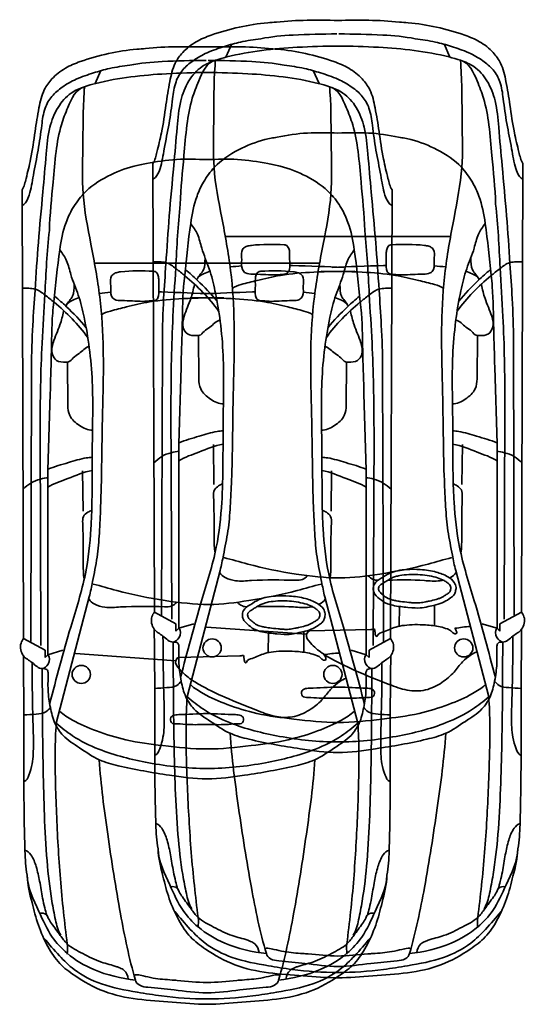
# Model space of a CAD drawing. Units: inches. Extents: x -24887 to 3061, y 1794 to 4919553.
# Tile 14 of 14: x -24887 to -22520, y 4914938 to 4919553. Entities that reach past the tile are written whole.
import ezdxf

# ---------------------------------------------------------------- set-up
doc = ezdxf.new("R2010")
doc.units = ezdxf.units.IN
doc.layers.add('door', color=4, linetype='Continuous', lineweight=25)
doc.layers.add('wall', color=7, linetype='Continuous', lineweight=35)

# ---------------------------------------------------------------- blocks, each defined once
blk = doc.blocks.new('A$C242571DA')
for p, q in [((1659.9, 1632), (1714.3, 1732.5)), ((1714.3, 1732.5), (3817.1, 1739.9)), ((1699.9, 1699.4), (2984.7, 1695.8)), ((1638.3, 1618.5), (1625.1, 1632)), ((1625.1, 1632), (1659.9, 1632)), ((1638.3, 1618.5), (2503.3, 1618.5)), ((1659.9, 1548.1), (1638.3, 1618.5)), ((1681.8, 1651.6), (2695.2, 1655.3)), ((2503.3, 1618.5), (2861.6, 1607.5)), ((1317.4, 1579.7), (1909.8, 1424.9)), ((3007.2, 1526.5), (2808.1, 1525.2)), ((1644, 1489.1), (1610.4, 1020.2)), ((2311.9, 1454.3), (2500.6, 1456.9)), ((3474.6, 1401.1), (3474.6, 843)), ((4315.2, 1398), (4377.3, 1370.5)), ((1626.1, 1006.5), (1632.8, 719.7)), ((3474.6, 345.6), (3474.6, 903.8)), ((1740.2, 584.9), (1649.3, 586.9)), ((1746.1, 420.6), (1649.3, 420.6)), ((4315.2, 348.7), (4377.3, 376.3)), ((1317.4, 167), (1909.8, 321.9)), ((2311.9, 292.5), (2500.6, 289.8)), ((1659.9, 198.7), (1638.3, 128.2)), ((3007.2, 220.3), (2808.1, 221.6)), ((2503.3, 128.2), (2861.6, 139.2)), ((1638.3, 128.2), (1625.1, 114.7)), ((1625.1, 114.7), (1659.9, 114.7)), ((1638.3, 128.2), (2503.3, 128.2)), ((1659.9, 114.7), (1714.3, 14.2)), ((1681.8, 95.1), (2695.2, 91.4)), ((1699.9, 47.3), (2984.7, 51)), ((1714.3, 14.2), (3817.1, 6.9))]:
    blk.add_line(p, q)
for centre in [(1546.4, 1462.5), (1546.4, 284.2)]:
    blk.add_ellipse(centre, major_axis=(0, 42.9), ratio=0.983266, start_param=4.712389, end_param=10.995574)
for points, knots in [([(0, 873.4), (0, 927.8), (15.6, 1088.6), (25.5, 1309.8), (120.7, 1476.4), (189.2, 1569), (273.5, 1623.1), (369.9, 1666.3), (483, 1694.7), (561.3, 1714.9), (604.6, 1715.7)], [0, 0, 0, 0, 0.16039, 0.479033, 0.632967, 0.722015, 0.817474, 0.927562, 1.03733, 1.167094, 1.167094, 1.167094, 1.167094]), ([(604.6, 1715.7), (545.5, 1714.5), (448.5, 1664.6), (320.8, 1610.6), (225.4, 1521.2), (147.3, 1390.5), (121.7, 1275.2), (113.6, 1208.7)], [0, 0, 0, 0, 0.1772572, 0.3124951, 0.4151678, 0.5597243, 0.7575412, 0.7575412, 0.7575412, 0.7575412]), ([(722.7, 1726.6), (720.8, 1714.9), (694.5, 1689.9), (643, 1671.8), (573.6, 1655.4), (508.5, 1647), (455.2, 1634.7), (428.7, 1627.3), (416.9, 1624.1)], [0, 0, 0, 0, 0.034703, 0.0959761, 0.1659336, 0.2471559, 0.2929944, 0.3295918, 0.3295918, 0.3295918, 0.3295918]), ([(604.6, 1715.7), (642.1, 1723.4), (788.5, 1729.2), (1039.3, 1732.2), (1344.5, 1729.9), (1542, 1733.1), (1633.8, 1733.7)], [0, 0, 0, 0, 0.114897, 0.437061, 0.754269, 1.029686, 1.029686, 1.029686, 1.029686]), ([(1043.6, 1729.2), (1048.6, 1717.9), (1080.9, 1704.2), (1138.6, 1687.6), (1237.7, 1685.6), (1394.7, 1691.3), (1521.7, 1692.4), (1601.5, 1692.7)], [0, 0, 0, 0, 0.0364992, 0.0923739, 0.1867837, 0.3273982, 0.5667068, 0.5667068, 0.5667068, 0.5667068]), ([(1356.8, 1732.2), (1357.1, 1712.8), (1360, 1678.8), (1363.9, 1630.5), (1383.3, 1613.5), (1391, 1607.2)], [0, 0, 0, 0, 1.462159, 2.651105, 3.386321, 3.386321, 3.386321, 3.386321]), ([(1714.3, 1732.5), (1707.7, 1737.6), (1683.3, 1753), (1628.7, 1741.2), (1605.6, 1691.5), (1561.7, 1652.4), (1594.1, 1610.3), (1627.9, 1608.3), (1638.3, 1618.5)], [0, 0, 0, 0, 0.024864, 0.0846267, 0.1362471, 0.1900683, 0.2245199, 0.2681841, 0.2681841, 0.2681841, 0.2681841]), ([(2414.7, 1735), (2424.9, 1723.3), (2447.2, 1698.8), (2461.2, 1657.6), (2468.1, 1629), (2468, 1616.1)], [1.808086, 1.808086, 1.808086, 1.808086, 2.918874, 4.131288, 5.10151, 5.10151, 5.10151, 5.10151]), ([(3356.5, 1739.4), (3354.9, 1719.2), (3360.8, 1678.2), (3324, 1631.5), (3255.4, 1544.3), (3187.1, 1476.2), (3125.2, 1432.2)], [0, 0, 0, 0, 0.0597371, 0.1139981, 0.1672498, 0.3938869, 0.3938869, 0.3938869, 0.3938869]), ([(3745.3, 1736.8), (3748.5, 1730.1), (3764.2, 1717.1), (3811.5, 1698.6), (3894.7, 1686.7), (4002.9, 1663.2), (4107.9, 1648.7), (4195.8, 1638.3), (4258.6, 1603.2), (4302.1, 1549.7), (4339.9, 1483.8), (4365.2, 1407.6), (4389.6, 1324.4), (4397.9, 1266.9), (4401.8, 1235.2)], [0, 0, 0, 0, 0.0219205, 0.0572122, 0.1522539, 0.2718866, 0.3894011, 0.4710097, 0.5346344, 0.5986698, 0.6733118, 0.758696, 0.8351341, 0.9293726, 0.9293726, 0.9293726, 0.9293726]), ([(3817.1, 1739.9), (3833.2, 1729.7), (3882.9, 1718.2), (3973.3, 1695.2), (4085.1, 1680.5), (4193.8, 1662.8), (4280.6, 1644.3), (4343.9, 1598.1), (4390, 1540.3), (4427.4, 1448.7), (4457.8, 1336.6), (4475.7, 1233.4), (4478.4, 1175.1), (4479.3, 1161.6)], [0, 0, 0, 0, 0.056668, 0.14946, 0.28161, 0.392935, 0.481686, 0.542967, 0.622845, 0.69797, 0.833643, 0.965665, 1.00577, 1.00577, 1.00577, 1.00577]), ([(2984.7, 1695.8), (3051, 1695.6), (3172.1, 1691.3), (3367.4, 1677.6), (3575.2, 1664.3), (3788.2, 1643.6), (3968, 1628.1), (4103.8, 1616.8), (4203.6, 1578.1), (4271.8, 1519.5), (4300.6, 1452.1), (4341.7, 1305.3), (4361.8, 1111.2), (4367.5, 936.8), (4367.5, 873.4)], [0, 0, 0, 0, 0.198873, 0.363323, 0.587433, 0.823543, 1.004622, 1.129816, 1.230113, 1.320655, 1.388577, 1.443334, 1.771447, 1.958652, 1.958652, 1.958652, 1.958652]), ([(310.7, 1637.3), (282.5, 1613.7), (230.1, 1569.9), (148.7, 1486.2), (84.8, 1361.3), (60, 1219), (32.6, 1054.3), (25.1, 944.9), (25.1, 873.4)], [0, 0, 0, 0, 0.1095129, 0.2035347, 0.3452507, 0.5161382, 0.6275464, 0.8383798, 0.8383798, 0.8383798, 0.8383798]), ([(426.8, 1656.7), (428.5, 1646.6), (426.9, 1625), (399.8, 1616.6), (368.1, 1593.9), (328, 1564.6), (271.6, 1523.9), (237, 1451.9), (196.2, 1376.7), (183.8, 1314.9), (170, 1279.6), (157.2, 1254.2), (133.3, 1244.4), (118.6, 1242.9)], [0, 0, 0, 0, 0.0304541, 0.0502818, 0.0786089, 0.1479133, 0.1986294, 0.2831705, 0.3780326, 0.4523267, 0.4667809, 0.4902599, 0.5347198, 0.5347198, 0.5347198, 0.5347198]), ([(323.7, 1557.5), (344.8, 1571.9), (400.4, 1585.1), (516, 1606.8), (680.3, 1625.8), (885.4, 1635.7), (1116.8, 1642.2), (1346.1, 1644.2), (1504.7, 1644.7), (1574, 1645.7)], [0, 0, 0, 0, 0.076148, 0.165903, 0.355672, 0.569871, 0.782325, 1.050047, 1.257936, 1.257936, 1.257936, 1.257936]), ([(1555.2, 1617.8), (1527.7, 1617.8), (1472.5, 1620.4), (1392.7, 1608.8), (1318.5, 1591), (1249.4, 1545.5), (1201.4, 1466.7), (1142.8, 1385.7), (1104.8, 1240.4), (1076, 1072.3), (1056.4, 932.4), (1056.4, 873.4)], [0, 0, 0, 0, 0.082256, 0.165174, 0.241383, 0.30939, 0.405348, 0.511507, 0.603349, 0.843635, 1.017671, 1.017671, 1.017671, 1.017671]), ([(1574, 1645.7), (1572.9, 1638), (1574.1, 1622), (1559.9, 1618.7), (1555.2, 1617.8)], [0, 0, 0, 0, 0.02274132, 0.03717479, 0.03717479, 0.03717479, 0.03717479]), ([(2424, 1618.7), (2441.5, 1589.9), (2464.2, 1518.9), (2495.4, 1450.9), (2501.6, 1411.3)], [0, 0, 0, 0, 0.1000351, 0.2184418, 0.2184418, 0.2184418, 0.2184418]), ([(2507.7, 1618.4), (2521, 1587.7), (2536.6, 1527.1), (2559.6, 1458.5), (2563.3, 1420.6), (2563.8, 1411.4)], [0, 0, 0, 0, 2.528586, 4.711885, 5.408215, 5.408215, 5.408215, 5.408215]), ([(2695.2, 1655.3), (2829.9, 1655.3), (3041.2, 1651.4), (3351.3, 1630.7), (3527.5, 1623.2), (3626.6, 1612)], [0, 0, 0, 0, 0.4042759, 0.6333827, 0.9326252, 0.9326252, 0.9326252, 0.9326252]), ([(1317.4, 1579.7), (1227.8, 1586.1), (1036, 1584.8), (741.2, 1572.5), (486.1, 1553.3), (333.3, 1534.3), (283.3, 1528.5)], [0, 0, 0, 0, 0.269375, 0.574535, 0.885339, 1.036319, 1.036319, 1.036319, 1.036319]), ([(1317.4, 1579.7), (1296.6, 1555.5), (1247.9, 1494.4), (1177.6, 1350.5), (1124.2, 1137.4), (1105.5, 964.9), (1105.5, 873.4)], [0, 0, 0, 0, 0.0947759, 0.2311242, 0.4700259, 0.7400315, 0.7400315, 0.7400315, 0.7400315]), ([(3535.9, 1563.1), (3520.1, 1550.9), (3484.4, 1526.1), (3408.2, 1510.9), (3323.4, 1473.1), (3207.9, 1445), (3072.6, 1422.2), (2866.9, 1404.6), (2626.4, 1412.9), (2396.7, 1410.8), (2200.9, 1416.9), (2001.3, 1438.2), (1732.1, 1525.9), (1527.9, 1578.9), (1407.5, 1610.7)], [0, 0, 0, 0, 0.05975, 0.126928, 0.230034, 0.336675, 0.482225, 0.641324, 0.954906, 1.203173, 1.330375, 1.542773, 1.802261, 2.175545, 2.175545, 2.175545, 2.175545]), ([(2861.6, 1607.5), (2921.1, 1607.3), (3047.2, 1600.8), (3191.4, 1602), (3356.6, 1584.1), (3498.3, 1570.6), (3623.2, 1549.4), (3664.1, 1533.3)], [0, 0, 0, 0, 0.1783018, 0.3787173, 0.431954, 0.6762374, 0.8077184, 0.8077184, 0.8077184, 0.8077184]), ([(3248.1, 1545.2), (3226.9, 1550.4), (3176.1, 1562.1), (3113.7, 1592.9), (3052.6, 1605.3), (3010.4, 1578.8), (3010.3, 1545.3), (3010.3, 1515.9), (3033.7, 1500.1), (3052.6, 1465.2), (3078.9, 1443.5), (3084, 1424.4)], [0, 0, 0, 0, 0.0655106, 0.1550445, 0.2094604, 0.2438604, 0.287164, 0.3001388, 0.3275984, 0.3616951, 0.4200969, 0.4200969, 0.4200969, 0.4200969]), ([(3319, 1587.1), (3303.3, 1568.1), (3256.9, 1516.7), (3206.7, 1467.3), (3171.4, 1439.5)], [0, 0, 0, 0, 1.868162, 5.271297, 5.271297, 5.271297, 5.271297]), ([(3626.6, 1612), (3702.5, 1609.1), (3826.2, 1596.8), (3991.4, 1583.2), (4111.7, 1562.4), (4212.2, 1522.7), (4290.4, 1488), (4300.7, 1447.5)], [0, 0, 0, 0, 0.2277977, 0.3719478, 0.4996814, 0.5863441, 0.709615, 0.709615, 0.709615, 0.709615]), ([(1372.8, 1563.1), (1357.2, 1545), (1321.6, 1490.1), (1277, 1385.7), (1232.8, 1244.2), (1211.1, 1069.4), (1196.8, 942.4), (1196.8, 873.4)], [0, 0, 0, 0, 0.0708922, 0.1925846, 0.3348457, 0.5072814, 0.7109928, 0.7109928, 0.7109928, 0.7109928]), ([(2808.1, 1525.2), (2791.9, 1525.1), (2751.9, 1519.7), (2710.6, 1472.6), (2690, 1431.1), (2690.5, 1409.6)], [0, 0, 0, 0, 0.0486628, 0.1144515, 0.1777721, 0.1777721, 0.1777721, 0.1777721]), ([(3275.5, 1532.8), (3287.5, 1528.3), (3299.8, 1504.9), (3308.4, 1482.5), (3311.7, 1472.6)], [0, 0, 0, 0, 0.983949, 1.771691, 1.771691, 1.771691, 1.771691]), ([(3372.2, 1495.3), (3354.4, 1496.8), (3316, 1494.7), (3291.6, 1525.8), (3275.5, 1532.8)], [0, 0, 0, 0, 0.0535488, 0.1060573, 0.1060573, 0.1060573, 0.1060573]), ([(3664.1, 1533.3), (3687, 1526), (3734.8, 1502.3), (3816.7, 1444.8), (3884.1, 1342.9), (3925.1, 1239.9), (3937.3, 1177), (3940.4, 1157.6)], [0, 0, 0, 0, 0.0720749, 0.1581284, 0.2958089, 0.4262456, 0.4842292, 0.4842292, 0.4842292, 0.4842292]), ([(1909.8, 1424.9), (1933.5, 1418.7), (1995.6, 1407.6), (2094.4, 1385.8), (2211.8, 1377.1), (2419, 1366.9), (2704.7, 1366.5), (3032.7, 1354.2), (3316.2, 1371), (3558.7, 1415.9), (3789.1, 1461.7), (4028.9, 1452.9), (4196.2, 1455.2), (4292.7, 1447.9), (4300.7, 1447.5)], [0, 0, 0, 0, 0.073325, 0.188896, 0.303039, 0.425821, 0.811242, 1.159737, 1.41058, 1.660623, 1.899627, 2.11145, 2.377727, 2.401703, 2.401703, 2.401703, 2.401703]), ([(1997.2, 1450.5), (2039.7, 1454.5), (2126.7, 1451.9), (2219.8, 1454.5), (2287.1, 1456.9), (2305.7, 1434.4), (2313.2, 1419.9), (2315.8, 1413.5)], [0, 0, 0, 0, 3.267856, 6.568708, 7.399663, 8.099385, 8.621705, 8.621705, 8.621705, 8.621705]), ([(1898.5, 1426.2), (1889, 1420.6), (1871, 1397.2), (1856.4, 1345.2), (1867.7, 1233.5), (1864.3, 1132.3), (1863, 1038.5), (1876.9, 1022.3), (1884.5, 1015.7)], [0, 0, 0, 0, 0.842998, 2.122875, 3.997599, 9.174838, 10.012722, 10.751336, 10.751336, 10.751336, 10.751336]), ([(1969.6, 1407.3), (1960.5, 1369.8), (1927, 1259.1), (1890.9, 1078.4), (1874.3, 933), (1874.3, 864.4)], [0, 0, 0, 0, 0.1139079, 0.3411539, 0.543502, 0.543502, 0.543502, 0.543502]), ([(113.6, 1208.7), (215.2, 1238.6), (443.2, 1284.9), (788, 1338.7), (1029.5, 1370.7), (1146.4, 1378.6)], [0, 0, 0, 0, 0.317374, 0.69576, 1.04714, 1.04714, 1.04714, 1.04714]), ([(3231.5, 1368.3), (3240.8, 1356.2), (3253.1, 1315.7), (3271.9, 1240.7), (3297.9, 1127.9), (3310.5, 974.6), (3311.2, 858.3), (3311.6, 794.4)], [0, 0, 0, 0, 0.0451009, 0.1211996, 0.2308505, 0.385263, 0.5739042, 0.5739042, 0.5739042, 0.5739042]), ([(3294.8, 1174.5), (3294.8, 1207.4), (3299.6, 1249.5), (3298.3, 1303.9), (3326.3, 1329), (3363.9, 1320.7), (3399.3, 1329.3), (3422.1, 1315.7), (3430.7, 1297.9), (3438.7, 1234.2), (3439.6, 1174.4), (3434.7, 1112.2), (3418.9, 1102), (3395.9, 1098.6), (3362.6, 1100.9), (3331.1, 1096.6), (3298.8, 1107.6), (3297.3, 1140.3), (3294.8, 1160.9), (3294.8, 1174.5)], [0, 0, 0, 0, 0.0969044, 0.1295913, 0.1506192, 0.1985921, 0.2360698, 0.2557908, 0.2719711, 0.2929882, 0.44406, 0.4519132, 0.4720918, 0.4918599, 0.5228758, 0.5707096, 0.5892096, 0.6145759, 0.654681, 0.654681, 0.654681, 0.654681]), ([(113.6, 1208.7), (103.3, 1207), (83.6, 1187.6), (76.5, 1122.2), (68.2, 1017.3), (53.4, 925), (53.4, 873.4)], [0, 0, 0, 0, 0.0314754, 0.0702057, 0.1915753, 0.3439346, 0.3439346, 0.3439346, 0.3439346]), ([(135.5, 1213.1), (139.1, 1211.8), (138.4, 1193.3), (132.6, 1168.3), (118.8, 1111.9), (115.6, 1058.9), (109, 974.6), (102.4, 920.1), (102.4, 873.4)], [0, 0, 0, 0, 0.0114788, 0.0403472, 0.0875838, 0.1755608, 0.1991501, 0.3369659, 0.3369659, 0.3369659, 0.3369659]), ([(4401.8, 1235.2), (4411.9, 1185.3), (4421.6, 1065.8), (4424.1, 946.5), (4424.1, 878)], [0, 0, 0, 0, 0.1502861, 0.3522699, 0.3522699, 0.3522699, 0.3522699]), ([(3940.4, 1157.6), (3949.9, 1111), (3964.3, 1016.4), (3960.5, 921), (3959.8, 873.4)], [0, 0, 0, 0, 0.140379, 0.2808468, 0.2808468, 0.2808468, 0.2808468]), ([(3339.2, 1099), (3339.1, 1094.8), (3336.4, 1010.6), (3333.2, 926.3), (3330, 846.2)], [11.235438, 11.235438, 11.235438, 11.235438, 11.552536, 17.586883, 17.586883, 17.586883, 17.586883]), ([(1311.3, 873.4), (1311.2, 902.4), (1309.2, 950.9), (1315, 1002.2), (1314.2, 1039.4), (1332.1, 1044.9), (1345.7, 1044.2), (1356.8, 1028.5), (1359.2, 970.2), (1361.5, 917.6), (1362.9, 873.4)], [0, 0, 0, 0, 0.0857277, 0.1381048, 0.1641986, 0.1769751, 0.1890325, 0.2028129, 0.2286049, 0.3592554, 0.3592554, 0.3592554, 0.3592554]), ([(1626.1, 1006.5), (1623.5, 1013), (1603.1, 1029.4), (1559.1, 995), (1523, 951.9), (1480.3, 878.3), (1430.5, 774.3), (1385.5, 658.5), (1343.7, 551.3), (1343, 461.7), (1380.3, 386.9), (1428.2, 329.9), (1480.1, 294.6), (1509.8, 257.4), (1524.8, 232.6), (1528, 222.1)], [0, 0, 0, 0, 0.527288, 1.647451, 3.487558, 5.099073, 7.968657, 12.238313, 14.475187, 16.613757, 18.744202, 20.639343, 22.223389, 23.452731, 24.286529, 24.286529, 24.286529, 24.286529]), ([(3231.5, 378.5), (3240.8, 390.5), (3253.1, 431), (3271.9, 506.1), (3297.9, 618.9), (3310.5, 772.1), (3311.2, 888.4), (3311.6, 952.4)], [0, 0, 0, 0, 0.0451009, 0.1211996, 0.2308505, 0.385263, 0.5739042, 0.5739042, 0.5739042, 0.5739042]), ([(3339.2, 647.8), (3339.1, 652), (3336.4, 736.2), (3333.2, 820.5), (3330, 900.6)], [11.235438, 11.235438, 11.235438, 11.235438, 11.552536, 17.586883, 17.586883, 17.586883, 17.586883]), ([(0, 873.4), (0, 819), (15.6, 658.1), (25.5, 437), (120.7, 270.3), (189.2, 177.8), (273.5, 123.7), (369.9, 80.4), (483, 52), (561.3, 31.9), (604.6, 31)], [0, 0, 0, 0, 0.16039, 0.479033, 0.632967, 0.722015, 0.817474, 0.927562, 1.03733, 1.167094, 1.167094, 1.167094, 1.167094]), ([(310.7, 109.5), (282.5, 133.1), (230.1, 176.9), (148.7, 260.5), (84.8, 385.5), (60, 527.8), (32.6, 692.4), (25.1, 801.9), (25.1, 873.4)], [0, 0, 0, 0, 0.1095129, 0.2035347, 0.3452507, 0.5161382, 0.6275464, 0.8383798, 0.8383798, 0.8383798, 0.8383798]), ([(113.6, 538.1), (103.3, 539.8), (83.6, 559.2), (76.5, 624.5), (68.2, 729.4), (53.4, 821.7), (53.4, 873.4)], [0, 0, 0, 0, 0.0314754, 0.0702057, 0.1915753, 0.3439346, 0.3439346, 0.3439346, 0.3439346]), ([(135.5, 533.6), (139.1, 534.9), (138.4, 553.4), (132.6, 578.4), (118.8, 634.9), (115.6, 687.8), (109, 772.2), (102.4, 826.7), (102.4, 873.4)], [0, 0, 0, 0, 0.0114788, 0.0403472, 0.0875838, 0.1755608, 0.1991501, 0.3369659, 0.3369659, 0.3369659, 0.3369659]), ([(1555.2, 129), (1527.7, 129), (1472.5, 126.3), (1392.7, 138), (1318.5, 155.7), (1249.4, 201.3), (1201.4, 280.1), (1142.8, 361.1), (1104.8, 506.4), (1076, 674.5), (1056.4, 814.4), (1056.4, 873.4)], [0, 0, 0, 0, 0.082256, 0.165174, 0.241383, 0.30939, 0.405348, 0.511507, 0.603349, 0.843635, 1.017671, 1.017671, 1.017671, 1.017671]), ([(1317.4, 167), (1296.6, 191.2), (1247.9, 252.4), (1177.6, 396.3), (1124.2, 609.4), (1105.5, 781.8), (1105.5, 873.4)], [0, 0, 0, 0, 0.0947759, 0.2311242, 0.4700259, 0.7400315, 0.7400315, 0.7400315, 0.7400315]), ([(1372.8, 183.6), (1357.2, 201.8), (1321.6, 256.7), (1277, 361), (1232.8, 502.6), (1211.1, 677.3), (1196.8, 804.3), (1196.8, 873.4)], [0, 0, 0, 0, 0.0708922, 0.1925846, 0.3348457, 0.5072814, 0.7109928, 0.7109928, 0.7109928, 0.7109928]), ([(1311.3, 873.4), (1311.2, 844.3), (1309.2, 795.8), (1315, 744.6), (1314.2, 707.4), (1332.1, 701.9), (1345.7, 702.6), (1356.8, 718.2), (1359.2, 776.6), (1361.5, 829.1), (1362.9, 873.4)], [0, 0, 0, 0, 0.0857277, 0.1381048, 0.1641986, 0.1769751, 0.1890325, 0.2028129, 0.2286049, 0.3592554, 0.3592554, 0.3592554, 0.3592554]), ([(1969.6, 339.5), (1960.5, 377), (1926.9, 487.6), (1892.9, 662.7), (1874.3, 801.8), (1874.3, 864.4)], [0, 0, 0, 0, 0.1139079, 0.3411539, 0.5260188, 0.5260188, 0.5260188, 0.5260188]), ([(2984.7, 51), (3051, 51.1), (3172.1, 55.5), (3367.4, 69.2), (3575.2, 82.5), (3788.2, 103.1), (3968, 118.7), (4103.8, 130), (4203.6, 168.6), (4271.8, 227.3), (4300.6, 294.7), (4341.7, 441.5), (4361.8, 635.5), (4367.5, 809.9), (4367.5, 873.4)], [0, 0, 0, 0, 0.198873, 0.363323, 0.587433, 0.823543, 1.004622, 1.129816, 1.230113, 1.320655, 1.388577, 1.443334, 1.771447, 1.958652, 1.958652, 1.958652, 1.958652]), ([(3940.4, 589.1), (3949.9, 635.7), (3964.3, 730.4), (3960.5, 825.8), (3959.8, 873.4)], [0, 0, 0, 0, 0.140379, 0.2808468, 0.2808468, 0.2808468, 0.2808468]), ([(4401.8, 511.5), (4411.9, 561.5), (4421.6, 681), (4424.1, 800.3), (4424.1, 868.8)], [0, 0, 0, 0, 0.1502861, 0.3522699, 0.3522699, 0.3522699, 0.3522699]), ([(1639.2, 326.1), (1635.3, 323.6), (1629, 318.4), (1613.1, 314.9), (1612, 324.2), (1613.2, 330.4), (1619, 337.5), (1629, 345.7), (1637.9, 366.1), (1649, 404.8), (1656.3, 472.9), (1656.2, 543.1), (1644.6, 610.9), (1623, 651.2), (1615, 684.3), (1598.5, 691.2), (1604, 696.6), (1610.3, 699.7), (1618.8, 698.9), (1625.9, 701.3), (1638.1, 698.6), (1633, 713.4), (1632.8, 719.7)], [0, 0, 0, 0, 0.0138597, 0.0278304, 0.0329137, 0.0379971, 0.0465756, 0.0592704, 0.0762214, 0.1105991, 0.1789801, 0.2766959, 0.3173629, 0.3800771, 0.4110544, 0.4160421, 0.4210284, 0.4277212, 0.4387433, 0.4448131, 0.4508005, 0.4694463, 0.4694463, 0.4694463, 0.4694463]), ([(1740.2, 584.9), (1737.8, 571.7), (1749.5, 644.3), (1766.4, 664.5), (1792.2, 700.2), (1821.5, 709.7), (1853.1, 703.9), (1874, 668.4), (1904.5, 622.6), (1915.6, 557.2), (1915.1, 484.2), (1905.7, 417.6), (1884.9, 362.8), (1859.3, 329.1), (1831.3, 318.1), (1810.8, 322.7), (1792.2, 329.3), (1777.9, 350.3), (1753, 385.9), (1737.9, 465.8), (1728.8, 497.3), (1742.4, 597.6), (1740.2, 584.9)], [0, 0, 0, 0, 0.03969, 0.089634, 0.13125, 0.1542862, 0.1797268, 0.2207266, 0.2680991, 0.3447665, 0.4095645, 0.4843001, 0.541515, 0.5817687, 0.6060665, 0.6262474, 0.6436722, 0.6634686, 0.6988791, 0.7758465, 0.8696394, 0.907731, 0.907731, 0.907731, 0.907731]), ([(1863.4, 685.6), (1863.6, 693.5), (1865.3, 711), (1876.9, 724.5), (1884.5, 731)], [9.436432, 9.436432, 9.436432, 9.436432, 10.012722, 10.751336, 10.751336, 10.751336, 10.751336]), ([(1764.9, 587), (1765.6, 590.8), (1766.4, 595.5), (1768.5, 605.7), (1769.7, 611.3), (1773.4, 626.6), (1775.6, 633), (1779.7, 642.1), (1781.6, 644.9), (1785.7, 650.6), (1787.1, 652.5), (1793, 660.3), (1797.4, 666.2), (1804.2, 673.7), (1806.8, 676.1), (1811.1, 679.4), (1812.9, 680.5), (1816.8, 682.1), (1818.8, 682.7), (1824.4, 683.5), (1828.3, 683.2), (1832.5, 682), (1833.6, 681.5), (1836, 680.2), (1837.9, 678.7), (1842.4, 673.7), (1844.9, 670.1), (1850.3, 661.7), (1853.4, 656.6), (1859.3, 647.3), (1862.1, 642.8), (1868.3, 632.6), (1871.4, 626.9), (1876.7, 615.7), (1878.9, 609.8), (1882.8, 597.4), (1884.4, 590.8), (1888.3, 570.5), (1889.7, 556.1), (1891.2, 527.4), (1891.1, 513.1), (1888.9, 470), (1885.1, 441.2), (1874.3, 404), (1870.6, 393.8), (1863.5, 378.7), (1860.6, 373.4), (1854.4, 363.6), (1851.2, 359.2), (1845, 352.6), (1842, 350.2), (1835.8, 346.4), (1832.6, 345.3), (1828.8, 344.6), (1827.9, 344.6), (1824.6, 344.9), (1822.6, 345.2), (1817.8, 346.4), (1814.9, 347.3), (1810.9, 348.7), (1809.4, 349.4), (1808.3, 350.1), (1808.1, 350.2), (1807.3, 351), (1806.7, 351.6), (1804.7, 354), (1803.1, 356.2), (1799.6, 361.3), (1798, 363.7), (1794.9, 368.2), (1793.4, 370.4), (1789.2, 376.9), (1786.7, 381), (1782.4, 389.3), (1780.5, 393.6), (1776.9, 403), (1775.2, 408), (1770.7, 423.5), (1768.3, 434.2), (1764.9, 450.5), (1763.6, 456.4), (1761.4, 466.8), (1760.4, 471.4), (1758.1, 484.4), (1757.3, 492.6), (1757.5, 510.7), (1757.8, 516.5), (1758.6, 528.4), (1759.1, 534.3), (1761.1, 553.9), (1763.1, 570.6), (1764.4, 581.5), (1764.6, 583), (1764.7, 585), (1764.8, 585.5), (1764.8, 586.5), (1764.8, 586.7), (1764.9, 587)], [0.497033, 0.497033, 0.497033, 0.497033, 0.723444, 0.723444, 0.974636, 0.974636, 1.50964, 1.50964, 2.044645, 2.044645, 2.271061, 2.271061, 2.862376, 2.862376, 3.217654, 3.217654, 3.537253, 3.537253, 3.856852, 3.856852, 4.368613, 4.368613, 4.584627, 4.584627, 4.99269, 4.99269, 5.400753, 5.400753, 5.808816, 5.808816, 6.216879, 6.216879, 6.778716, 6.778716, 7.350371, 7.350371, 7.922025, 7.922025, 9.065335, 9.065335, 10.208644, 10.208644, 12.495263, 12.495263, 13.409896, 13.409896, 13.929088, 13.929088, 14.44828, 14.44828, 14.909885, 14.909885, 15.371489, 15.371489, 15.62524, 15.62524, 15.87899, 15.87899, 16.120875, 16.120875, 16.36276, 16.36276, 16.51635, 16.51635, 16.669941, 16.669941, 16.921521, 16.921521, 17.136676, 17.136676, 17.351831, 17.351831, 17.782142, 17.782142, 18.204974, 18.204974, 18.627807, 18.627807, 19.473473, 19.473473, 19.978923, 19.978923, 20.484372, 20.484372, 21.475119, 21.475119, 21.859144, 21.859144, 22.162884, 22.162884, 22.770362, 22.770362, 22.900493, 22.900493, 22.951221, 22.951221, 22.964298, 22.964298, 22.964298, 22.964298]), ([(3294.8, 572.3), (3294.8, 539.4), (3299.6, 497.2), (3298.3, 442.9), (3326.3, 417.8), (3363.9, 426), (3399.3, 417.5), (3422.1, 431), (3430.7, 448.9), (3438.7, 512.5), (3439.6, 572.4), (3434.7, 634.6), (3418.9, 644.7), (3395.9, 648.2), (3362.6, 645.9), (3331.1, 650.1), (3298.8, 639.2), (3297.3, 606.5), (3294.8, 585.9), (3294.8, 572.3)], [0, 0, 0, 0, 0.0969044, 0.1295913, 0.1506192, 0.1985921, 0.2360698, 0.2557908, 0.2719711, 0.2929882, 0.44406, 0.4519132, 0.4720918, 0.4918599, 0.5228758, 0.5707096, 0.5892096, 0.6145759, 0.654681, 0.654681, 0.654681, 0.654681]), ([(1863.7, 379.4), (1862.6, 384.2), (1857.6, 413.7), (1866.5, 501.6), (1865.2, 581.4), (1864.1, 639.5)], [1.749253, 1.749253, 1.749253, 1.749253, 2.122875, 3.997599, 8.307432, 8.307432, 8.307432, 8.307432]), ([(3664.1, 213.5), (3687, 220.8), (3734.8, 244.4), (3816.7, 302), (3884.1, 403.8), (3925.1, 506.9), (3937.3, 569.7), (3940.4, 589.1)], [0, 0, 0, 0, 0.0720749, 0.1581284, 0.2958089, 0.4262456, 0.4842292, 0.4842292, 0.4842292, 0.4842292]), ([(3817.1, 6.9), (3833.2, 17), (3882.9, 28.6), (3973.3, 51.5), (4085.1, 66.3), (4193.8, 84), (4280.6, 102.4), (4343.9, 148.6), (4390, 206.4), (4427.4, 298), (4457.8, 410.1), (4475.7, 513.3), (4478.4, 571.6), (4479.3, 585.2)], [0, 0, 0, 0, 0.056668, 0.14946, 0.28161, 0.392935, 0.481686, 0.542967, 0.622845, 0.69797, 0.833643, 0.965665, 1.00577, 1.00577, 1.00577, 1.00577]), ([(604.6, 31), (545.5, 32.3), (448.5, 82.2), (320.8, 136.1), (225.4, 225.5), (147.3, 356.2), (121.7, 471.5), (113.6, 538.1)], [0, 0, 0, 0, 0.1772572, 0.3124951, 0.4151678, 0.5597243, 0.7575412, 0.7575412, 0.7575412, 0.7575412]), ([(113.6, 538.1), (215.2, 508.2), (443.2, 461.9), (788, 408.1), (1029.5, 376), (1146.4, 368.2)], [0, 0, 0, 0, 0.317374, 0.69576, 1.04714, 1.04714, 1.04714, 1.04714]), ([(3745.3, 10), (3748.5, 16.7), (3764.2, 29.7), (3811.5, 48.1), (3894.7, 60.1), (4002.9, 83.6), (4107.9, 98), (4195.8, 108.4), (4258.6, 143.5), (4302.1, 197), (4339.9, 262.9), (4365.2, 339.2), (4389.6, 422.4), (4397.9, 479.8), (4401.8, 511.5)], [0, 0, 0, 0, 0.0219205, 0.0572122, 0.1522539, 0.2718866, 0.3894011, 0.4710097, 0.5346344, 0.5986698, 0.6733118, 0.758696, 0.8351341, 0.9293726, 0.9293726, 0.9293726, 0.9293726]), ([(426.8, 90), (428.5, 100.2), (426.9, 121.8), (399.8, 130.1), (368.1, 152.8), (328, 182.2), (271.6, 222.8), (237, 294.9), (196.2, 370.1), (183.8, 431.9), (170, 467.2), (157.2, 492.6), (133.3, 502.4), (118.6, 503.9)], [0, 0, 0, 0, 0.0304541, 0.0502818, 0.0786089, 0.1479133, 0.1986294, 0.2831705, 0.3780326, 0.4523267, 0.4667809, 0.4902599, 0.5347198, 0.5347198, 0.5347198, 0.5347198]), ([(1909.8, 321.9), (1933.5, 328.1), (1995.6, 339.2), (2094.4, 361), (2211.8, 369.6), (2419, 379.8), (2704.7, 380.3), (3032.7, 392.6), (3316.2, 375.8), (3558.7, 330.9), (3789.1, 285.1), (4028.9, 293.9), (4196.2, 291.5), (4292.7, 298.8), (4300.7, 299.2)], [0, 0, 0, 0, 0.073325, 0.188896, 0.303039, 0.425821, 0.811242, 1.159737, 1.41058, 1.660623, 1.899627, 2.11145, 2.377727, 2.401703, 2.401703, 2.401703, 2.401703]), ([(3535.9, 183.7), (3520.1, 195.9), (3484.4, 220.6), (3408.2, 235.8), (3323.4, 273.7), (3207.9, 301.8), (3072.6, 324.6), (2866.9, 342.1), (2626.4, 333.8), (2396.7, 335.9), (2200.9, 329.9), (2001.3, 308.6), (1732.1, 220.8), (1527.9, 167.8), (1407.5, 136)], [0, 0, 0, 0, 0.05975, 0.126928, 0.230034, 0.336675, 0.482225, 0.641324, 0.954906, 1.203173, 1.330375, 1.542773, 1.802261, 2.175545, 2.175545, 2.175545, 2.175545]), ([(1898.5, 320.6), (1889, 326.2), (1880.8, 336.8), (1874.8, 348.3), (1874, 349.7)], [0, 0, 0, 0, 0.8429982, 0.9626806, 0.9626806, 0.9626806, 0.9626806]), ([(1997.2, 296.3), (2039.7, 292.2), (2126.7, 294.9), (2219.8, 292.3), (2287.1, 289.9), (2305.7, 312.3), (2313.2, 326.9), (2315.8, 333.2)], [0, 0, 0, 0, 3.267856, 6.568708, 7.399663, 8.099385, 8.621705, 8.621705, 8.621705, 8.621705]), ([(2424, 128), (2441.5, 156.9), (2464.2, 227.8), (2495.4, 295.8), (2501.6, 335.5)], [0, 0, 0, 0, 0.1000351, 0.2184418, 0.2184418, 0.2184418, 0.2184418]), ([(2507.7, 128.3), (2521, 159.1), (2536.6, 219.7), (2559.6, 288.3), (2563.3, 326.1), (2563.8, 335.3)], [0, 0, 0, 0, 2.528586, 4.711885, 5.408215, 5.408215, 5.408215, 5.408215]), ([(2808.1, 221.6), (2791.9, 221.6), (2751.9, 227.1), (2710.6, 274.2), (2690, 315.7), (2690.5, 337.1)], [0, 0, 0, 0, 0.0486628, 0.1144515, 0.1777721, 0.1777721, 0.1777721, 0.1777721]), ([(3248.1, 201.6), (3226.9, 196.3), (3176.1, 184.7), (3113.7, 153.8), (3052.6, 141.4), (3010.4, 168), (3010.3, 201.5), (3010.3, 230.9), (3033.7, 246.6), (3052.6, 281.6), (3078.9, 303.2), (3084, 322.4)], [0, 0, 0, 0, 0.0655106, 0.1550445, 0.2094604, 0.2438604, 0.287164, 0.3001388, 0.3275984, 0.3616951, 0.4200969, 0.4200969, 0.4200969, 0.4200969]), ([(3356.5, 7.4), (3354.9, 27.5), (3360.8, 68.5), (3324, 115.2), (3255.4, 202.5), (3187.1, 270.5), (3125.2, 314.6)], [0, 0, 0, 0, 0.0597371, 0.1139981, 0.1672498, 0.3938869, 0.3938869, 0.3938869, 0.3938869]), ([(3319, 159.7), (3303.3, 178.6), (3256.9, 230), (3206.7, 279.5), (3171.4, 307.2)], [0, 0, 0, 0, 1.868162, 5.271297, 5.271297, 5.271297, 5.271297]), ([(3626.6, 134.7), (3702.5, 137.7), (3826.2, 149.9), (3991.4, 163.5), (4111.7, 184.4), (4212.2, 224.1), (4290.4, 258.8), (4300.7, 299.2)], [0, 0, 0, 0, 0.2277977, 0.3719478, 0.4996814, 0.5863441, 0.709615, 0.709615, 0.709615, 0.709615]), ([(3275.5, 214), (3287.5, 218.5), (3299.8, 241.9), (3308.4, 264.3), (3311.7, 274.2)], [0, 0, 0, 0, 0.983949, 1.771691, 1.771691, 1.771691, 1.771691]), ([(3372.2, 251.5), (3354.4, 249.9), (3316, 252), (3291.6, 220.9), (3275.5, 214)], [0, 0, 0, 0, 0.0535488, 0.1060573, 0.1060573, 0.1060573, 0.1060573]), ([(1317.4, 167), (1227.8, 160.7), (1036, 161.9), (741.2, 174.2), (486.1, 193.4), (333.3, 212.5), (283.3, 218.3)], [0, 0, 0, 0, 0.269375, 0.574535, 0.885339, 1.036319, 1.036319, 1.036319, 1.036319]), ([(323.7, 189.2), (344.8, 174.9), (400.4, 161.7), (516, 139.9), (680.3, 121), (885.4, 111), (1116.8, 104.5), (1346.1, 102.5), (1504.7, 102), (1574, 101.1)], [0, 0, 0, 0, 0.076148, 0.165903, 0.355672, 0.569871, 0.782325, 1.050047, 1.257936, 1.257936, 1.257936, 1.257936]), ([(2861.6, 139.2), (2921.1, 139.4), (3047.2, 146), (3191.4, 144.8), (3356.6, 162.6), (3498.3, 176.1), (3623.2, 197.4), (3664.1, 213.5)], [0, 0, 0, 0, 0.1783018, 0.3787173, 0.431954, 0.6762374, 0.8077184, 0.8077184, 0.8077184, 0.8077184]), ([(1356.8, 14.5), (1357.1, 33.9), (1360, 68), (1363.9, 116.3), (1383.3, 133.2), (1391, 139.5)], [0, 0, 0, 0, 1.462159, 2.651105, 3.386321, 3.386321, 3.386321, 3.386321]), ([(1714.3, 14.2), (1707.7, 9.2), (1683.3, -6.3), (1628.7, 5.5), (1605.6, 55.3), (1561.7, 94.4), (1594.1, 136.5), (1627.9, 138.5), (1638.3, 128.2)], [0, 0, 0, 0, 0.024864, 0.0846267, 0.1362471, 0.1900683, 0.2245199, 0.2681841, 0.2681841, 0.2681841, 0.2681841]), ([(722.7, 20.2), (720.8, 31.8), (694.5, 56.8), (643, 75), (573.6, 91.4), (508.5, 99.8), (455.2, 112.1), (428.7, 119.5), (416.9, 122.6)], [0, 0, 0, 0, 0.034703, 0.0959761, 0.1659336, 0.2471559, 0.2929944, 0.3295918, 0.3295918, 0.3295918, 0.3295918]), ([(1574, 101.1), (1572.9, 108.7), (1574.1, 124.8), (1559.9, 128), (1555.2, 129)], [0, 0, 0, 0, 0.02274132, 0.03717479, 0.03717479, 0.03717479, 0.03717479]), ([(2414.7, 11.8), (2424.9, 23.5), (2447.2, 48), (2461.2, 89.1), (2468.1, 117.8), (2468, 130.7)], [1.808086, 1.808086, 1.808086, 1.808086, 2.918874, 4.131288, 5.10151, 5.10151, 5.10151, 5.10151]), ([(2695.2, 91.4), (2829.9, 91.5), (3041.2, 95.4), (3351.3, 116.1), (3527.5, 123.5), (3626.6, 134.7)], [0, 0, 0, 0, 0.4042759, 0.6333827, 0.9326252, 0.9326252, 0.9326252, 0.9326252]), ([(1043.6, 17.6), (1048.6, 28.9), (1080.9, 42.6), (1138.6, 59.2), (1237.7, 61.2), (1394.7, 55.4), (1521.7, 54.3), (1601.5, 54.1)], [0, 0, 0, 0, 0.0364992, 0.0923739, 0.1867837, 0.3273982, 0.5667068, 0.5667068, 0.5667068, 0.5667068]), ([(604.6, 31), (642.1, 23.4), (788.5, 17.5), (1039.3, 14.6), (1344.5, 16.8), (1542, 13.6), (1633.8, 13.1)], [0, 0, 0, 0, 0.114897, 0.437061, 0.754269, 1.029686, 1.029686, 1.029686, 1.029686])]:
    blk.add_open_spline(points, degree=3, knots=knots)
for points in [[(283.3, 1528.5), (267.8, 1524.6), (251.4, 1527.5), (235.4, 1528.5)], [(3331.9, 1378.1), (3334.2, 1360.4), (3335.9, 1342.5), (3337.3, 1324.5)], [(4479.3, 1161.6), (4491, 1066.2), (4488, 969.5), (4488, 873.4)], [(4479.3, 585.2), (4491, 680.6), (4488, 777.3), (4488, 873.4)], [(3331.9, 368.6), (3334.2, 386.4), (3335.9, 404.3), (3337.3, 422.2)], [(1646.2, 253.1), (1647.8, 277.5), (1640, 301.6), (1639.2, 326.1)], [(283.3, 218.3), (267.8, 222.1), (251.4, 219.2), (235.4, 218.3)]]:
    blk.add_open_spline(points, degree=3)
blk = doc.blocks.new('CAR')
blk.add_blockref('A$C242571DA', (-29.4, -512.9))
blk = doc.blocks.new('new block')
blk.add_blockref('CAR', (4912883, 25875.5))
blk = doc.blocks.new('2.6door')
at = {"layer": 'wall'}
blk.add_blockref('new block', (0, 0), dxfattribs=at)

msp = doc.modelspace()

# ---------------------------------------------------------------- block references
at = {"layer": 'door', "rotation": 90}
for p in [(2838.93, 2207.94), (2838.93, 2207.94), (2225.92, 2083.94), (2225.92, 2083.94)]:
    msp.add_blockref('2.6door', p, dxfattribs=at)

doc.saveas('drawing.dxf')
